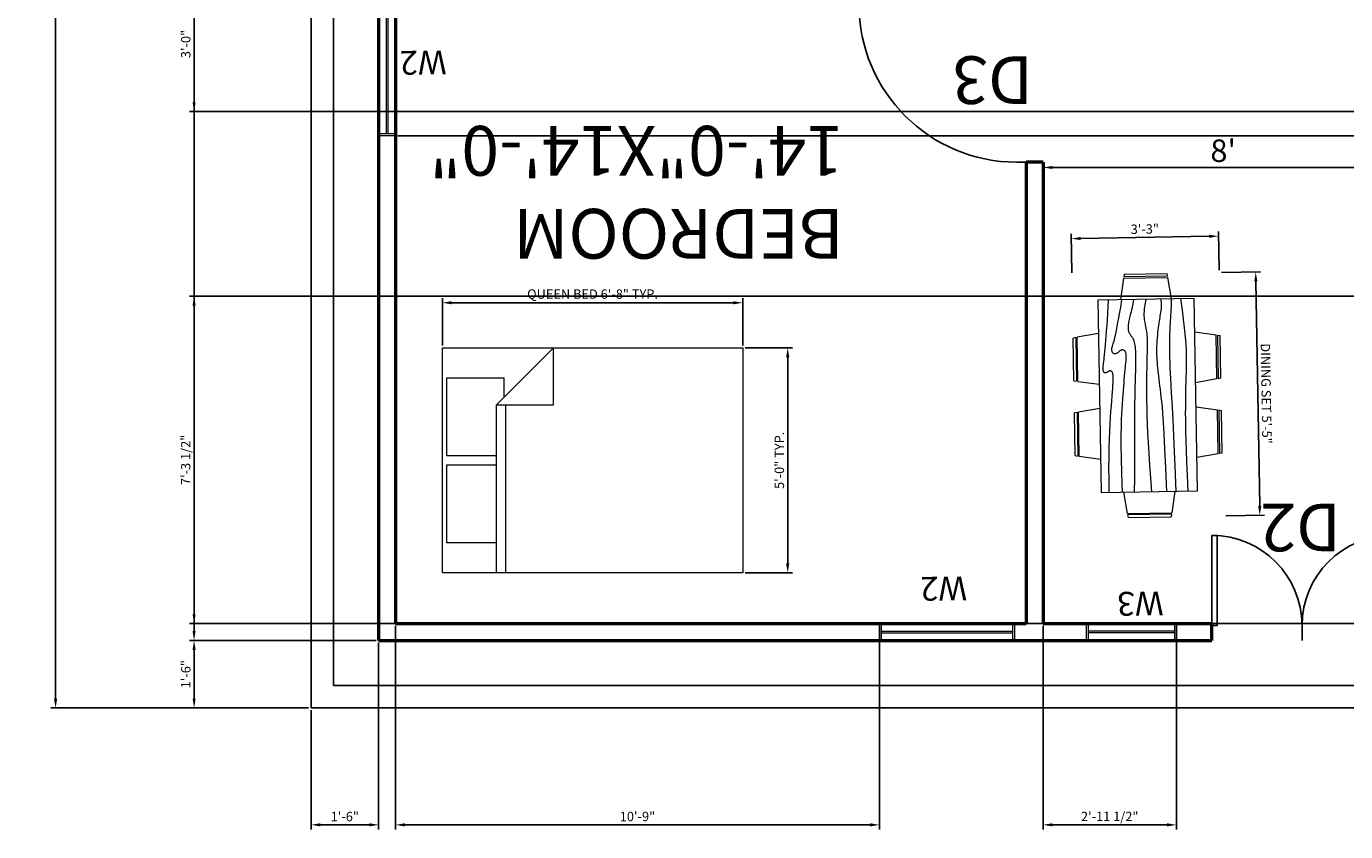
# Model space of a CAD drawing. Units: inches. Extents: x 1989 to 2637, y 1032 to 1611.
# Tile 1 of 5: x 1989 to 2340, y 1032 to 1247. Entities that reach past the tile are written whole.
import ezdxf

# ---------------------------------------------------------------- set-up
doc = ezdxf.new("R2010")
doc.units = ezdxf.units.IN
for name, color, linetype, lineweight in [('A-ANNO-TEXT', 1, 'Continuous', 18), ('A-AREA-IDEN', 1, 'Continuous', 25), ('C-PROP', 7, 'Continuous', 25), ('DIMENSIONS', 7, 'Continuous', 18), ('doors', 5, 'Continuous', 25), ('furniture', 8, 'Continuous', 18), ('walls', 7, 'Continuous', 50), ('windows', 3, 'Continuous', 18)]:
    doc.layers.add(name, color=color, linetype=linetype, lineweight=lineweight)
doc.styles.get("Standard").update_dxf_attribs({"font": 'arial.ttf'})
doc.dimstyles.new('ISO-25', dxfattribs={"dimtxt": 2.5, "dimasz": 2.5, "dimexe": 1.25, "dimexo": 0.625, "dimtad": 1, "dimlunit": 4, "dimtxsty": 'Standard', "dimcen": 2.5, "dimadec": 0, "dimazin": 0, "dimtfac": 1, "dimtmove": 0, "dimatfit": 3, "dimfxl": 1, "dimarcsym": 0})

# ---------------------------------------------------------------- blocks, each defined once
blk = doc.blocks.new('*U2')
for p, q in [((0, 0), (0, -5)), ((30, 0), (30, -5))]:
    blk.add_line(p, q)
blk.add_lwpolyline([(0, 0), (0, 30), (1.75, 30), (1.75, 0)], close=True)
blk.add_arc((0, 0), 30, 0, 90)
blk = doc.blocks.new('Dining Set - 36 x 72 in.')
for p, q in [((-22.2343, 26.00059), (-23.4847, 17.99762)), ((-22.2304, 26), (-5.7608, 26)), ((-22, 27.5), (-22.1562, 26.50042)), ((-5.8416, 26.5), (-22.1534, 26.5)), ((-22, 27.5), (-6, 27.5)), ((-5.8437, 26.49966), (-6, 27.5)), ((-4.5152, 17.99762), (-5.7655, 25.99926)), ((5.7657, 26.00059), (4.5153, 17.99762)), ((5.7696, 26), (22.2392, 26)), ((6, 27.5), (5.8438, 26.50042)), ((22.1584, 26.5), (5.8466, 26.5)), ((6, 27.5), (22, 27.5)), ((22.1563, 26.49966), (22, 27.5)), ((23.4848, 17.99762), (22.2345, 25.99926)), ((36, 18), (-36, 18)), ((-36, 18), (-36, -18)), ((36, -18), (36, 18)), ((-45.5, 8), (-44.5004, 8.15617)), ((-45.5, 8), (-45.5, -8)), ((-44.5, -8.15843), (-44.5, 8.15338)), ((-44.0006, 8.23428), (-35.9976, 9.48474)), ((-44, 8.23041), (-44, -8.23915)), ((44.0006, 8.23428), (35.9976, 9.48474)), ((44, 8.23041), (44, -8.23915)), ((44.5, -8.15843), (44.5, 8.15338)), ((45.5, 8), (44.5005, 8.15617)), ((45.5, 8), (45.5, -8)), ((-44.4997, -8.15631), (-45.5, -8)), ((-35.9976, -9.48476), (-43.9993, -8.2345)), ((35.9976, -9.48476), (43.9993, -8.2345)), ((44.4997, -8.15631), (45.5, -8)), ((-36, -18), (36, -18)), ((-22.2343, -26.0006), (-23.4847, -17.99762)), ((-4.5152, -17.99762), (-5.7655, -25.99928)), ((5.7657, -26.0006), (4.5153, -17.99762)), ((23.4848, -17.99762), (22.2345, -25.99928)), ((-22.2304, -26), (-5.7608, -26)), ((-22, -27.5), (-22.1562, -26.50044)), ((-5.8416, -26.5), (-22.1534, -26.5)), ((-22, -27.5), (-6, -27.5)), ((-5.8437, -26.49967), (-6, -27.5)), ((5.7696, -26), (22.2392, -26)), ((6, -27.5), (5.8438, -26.50044)), ((22.1584, -26.5), (5.8466, -26.5)), ((6, -27.5), (22, -27.5)), ((22.1563, -26.49967), (22, -27.5))]:
    blk.add_line(p, q)
for points in [[(-36, 15), (-31.1772, 14.97754), (-26.8079, 14.91406), (-22.8538, 14.81543), (-19.276, 14.6875), (-16.0362, 14.53613), (-13.0957, 14.36718), (-10.4159, 14.18652), (-7.9583, 14), (-5.6904, 13.81315), (-3.6035, 13.63021), (-1.6954, 13.45508), (0.0365, 13.29166), (1.5945, 13.14388), (2.9811, 13.01562), (4.1988, 12.9108), (5.25, 12.83333), (6.1393, 12.78613), (6.8802, 12.76823), (7.4883, 12.77767), (7.9792, 12.8125), (8.3685, 12.87077), (8.6719, 12.95052), (8.9049, 13.0498), (9.0833, 13.16666), (9.2205, 13.29899), (9.3216, 13.44401), (9.3895, 13.59879), (9.4271, 13.76041), (9.4373, 13.92594), (9.4232, 14.09245), (9.3875, 14.257), (9.3333, 14.41666), (9.2638, 14.56917), (9.1836, 14.71484), (9.0975, 14.85465), (9.0104, 14.98958), (8.9272, 15.1206), (8.8529, 15.2487), (8.7922, 15.37483), (8.75, 15.5), (8.7305, 15.62467), (8.7344, 15.74739), (8.7617, 15.86621), (8.8125, 15.97916), (8.8867, 16.08431), (8.9844, 16.17968), (9.1055, 16.26334), (9.25, 16.33333), (9.4189, 16.38802), (9.6172, 16.42708), (9.8506, 16.45052), (10.125, 16.45833), (10.4463, 16.45052), (10.8203, 16.42708), (11.2529, 16.38802), (11.75, 16.33333), (12.3184, 16.26318), (12.9694, 16.17838), (13.7151, 16.07991), (14.5677, 15.96875), (15.5395, 15.84586), (16.6426, 15.71224), (17.8893, 15.56884), (19.2917, 15.41666), (20.859, 15.25667), (22.5879, 15.08984), (24.4721, 14.91715), (26.5052, 14.73958), (28.6809, 14.5581), (30.9929, 14.3737), (33.4347, 14.18733), (36, 14)], [(-36, 10), (-28.9766, 10.14274), (-23.1725, 10.20442), (-18.4241, 10.19775), (-14.5677, 10.13541), (-11.4399, 10.03011), (-8.877, 9.89453), (-6.7154, 9.74137), (-4.7917, 9.58333), (-2.9698, 9.43082), (-1.2246, 9.28515), (0.4415, 9.14534), (2.026, 9.01041), (3.5266, 8.87939), (4.9408, 8.7513), (6.266, 8.62516), (7.5, 8.5), (8.6411, 8.37549), (9.6914, 8.2539), (10.6538, 8.13818), (11.5312, 8.03125), (12.3267, 7.93603), (13.043, 7.85547), (13.6831, 7.79248), (14.25, 7.75), (14.7471, 7.7303), (15.1797, 7.73307), (15.5537, 7.75732), (15.875, 7.80208), (16.1494, 7.86637), (16.3828, 7.94922), (16.5811, 8.04964), (16.75, 8.16666), (16.8944, 8.29915), (17.0143, 8.44531), (17.1089, 8.60319), (17.1771, 8.77083), (17.218, 8.94629), (17.2305, 9.1276), (17.2137, 9.31282), (17.1667, 9.5), (17.0895, 9.6875), (16.987, 9.875), (16.8649, 10.0625), (16.7292, 10.25), (16.5856, 10.4375), (16.4401, 10.625), (16.2985, 10.8125), (16.1667, 11), (16.05, 11.18733), (15.9518, 11.3737), (15.8752, 11.5581), (15.8229, 11.73958), (15.798, 11.91715), (15.8034, 12.08984), (15.842, 12.25667), (15.9167, 12.41666), (16.0295, 12.56836), (16.1784, 12.70833), (16.3605, 12.83268), (16.5729, 12.9375), (16.8127, 13.01888), (17.0768, 13.07291), (17.3625, 13.0957), (17.6667, 13.08333), (17.9894, 13.03312), (18.3418, 12.94726), (18.7382, 12.82918), (19.1927, 12.68229), (19.7195, 12.51001), (20.3327, 12.31575), (21.0465, 12.10294), (21.875, 11.875), (22.8357, 11.63354), (23.959, 11.37304), (25.2786, 11.08618), (26.8282, 10.76562), (28.6414, 10.40405), (30.752, 9.99414), (33.1936, 9.52856), (36, 9)], [(-36, 5.5), (-30.7157, 5.3348), (-26.069, 5.20963), (-21.9946, 5.11767), (-18.4271, 5.05208), (-15.3009, 5.00602), (-12.5508, 4.97265), (-10.1112, 4.94515), (-7.9167, 4.91666), (-5.909, 4.88167), (-4.0586, 4.83984), (-2.3429, 4.79215), (-0.7396, 4.73958), (0.7739, 4.6831), (2.22, 4.6237), (3.6213, 4.56233), (5, 4.5), (6.373, 4.43782), (7.7344, 4.3776), (9.0723, 4.32129), (10.375, 4.27083), (11.6309, 4.22819), (12.8281, 4.19531), (13.9551, 4.17415), (15, 4.16666), (15.954, 4.17448), (16.819, 4.19791), (17.6001, 4.23698), (18.3021, 4.29166), (18.9299, 4.36198), (19.4883, 4.44791), (19.9823, 4.54948), (20.4167, 4.66666), (20.7969, 4.79899), (21.1302, 4.94401), (21.4245, 5.09879), (21.6875, 5.26041), (21.9271, 5.42594), (22.1511, 5.59245), (22.3672, 5.757), (22.5834, 5.91666), (22.8065, 6.06868), (23.0404, 6.21093), (23.2879, 6.34147), (23.5521, 6.45833), (23.8358, 6.55957), (24.142, 6.64323), (24.4735, 6.70735), (24.8334, 6.75), (25.2235, 6.76969), (25.642, 6.76692), (26.0858, 6.74267), (26.5521, 6.69791), (27.0379, 6.63362), (27.5404, 6.55078), (28.0565, 6.45036), (28.5834, 6.33333), (29.1242, 6.19987), (29.7071, 6.04687), (30.3661, 5.87044), (31.1354, 5.66666), (32.0493, 5.43164), (33.142, 5.16146), (34.4475, 4.85221), (36, 4.5)], [(-36, -1), (-30.7915, -0.6591), (-26.0195, -0.38216), (-21.6519, -0.16284), (-17.6563, 0.00521), (-14.0005, 0.12833), (-10.6523, 0.21289), (-7.5796, 0.26522), (-4.75, 0.29166), (-2.134, 0.29793), (0.2878, 0.28711), (2.5317, 0.26163), (4.6146, 0.22396), (6.5529, 0.17651), (8.3633, 0.12174), (10.0623, 0.06209), (11.6667, 0), (13.1899, -0.06201), (14.6341, -0.1211), (15.9982, -0.17432), (17.2813, -0.21875), (18.4823, -0.25147), (19.6003, -0.26953), (20.6343, -0.27002), (21.5834, -0.25), (22.4481, -0.20768), (23.2357, -0.14584), (23.9549, -0.06836), (24.6146, 0.02083), (25.2235, 0.11784), (25.7904, 0.21875), (26.3241, 0.31966), (26.8334, 0.41666), (27.3265, 0.50618), (27.8099, 0.58593), (28.2894, 0.65397), (28.7709, 0.70833), (29.2601, 0.74707), (29.763, 0.76823), (30.2855, 0.76985), (30.8334, 0.75), (31.4088, 0.70784), (31.9994, 0.64713), (32.589, 0.57275), (33.1615, 0.48958), (33.7008, 0.4025), (34.1908, 0.3164), (34.6153, 0.23616), (34.9584, 0.16666), (35.2099, 0.11165), (35.3848, 0.07031), (35.504, 0.04069), (35.5886, 0.02083), (35.6594, 0.00879), (35.7377, 0.0026), (35.8442, 0.00032), (36, 0)], [(-36, -6.5), (-27.1843, -6.31267), (-20.084, -6.1263), (-14.469, -5.9419), (-10.1094, -5.76042), (-6.7752, -5.58285), (-4.2363, -5.41016), (-2.2629, -5.24333), (-0.625, -5.08334), (0.8708, -4.93099), (2.2715, -4.78646), (3.5872, -4.64974), (4.8281, -4.52084), (6.0046, -4.39974), (7.127, -4.28646), (8.2053, -4.18099), (9.25, -4.08334), (10.2705, -3.99382), (11.2734, -3.91407), (12.2647, -3.84603), (13.25, -3.79167), (14.2354, -3.75293), (15.2266, -3.73177), (16.2295, -3.73015), (17.25, -3.75), (18.2912, -3.79248), (19.3451, -3.85547), (20.4009, -3.93604), (21.4479, -4.03125), (22.4754, -4.13819), (23.4727, -4.25391), (24.4289, -4.37549), (25.3334, -4.5), (26.1785, -4.62492), (26.9694, -4.74935), (27.7145, -4.87281), (28.4219, -4.99479), (29.1, -5.11483), (29.7572, -5.23242), (30.4016, -5.34709), (31.0417, -5.45834), (31.6837, -5.56437), (32.3262, -5.65821), (32.9658, -5.73153), (33.599, -5.77604), (34.2224, -5.78345), (34.8327, -5.74545), (35.4264, -5.65373), (36, -5.5)], [(-36, -10), (-26.4022, -9.81299), (-18.4675, -9.62891), (-11.9839, -9.45069), (-6.7396, -9.28125), (-2.5226, -9.12354), (0.8789, -8.98047), (3.6769, -8.85498), (6.0833, -8.75), (8.2767, -8.66765), (10.3021, -8.60677), (12.1712, -8.56543), (13.8958, -8.54167), (15.4876, -8.53353), (16.9583, -8.53907), (18.3197, -8.55632), (19.5834, -8.58334), (20.7616, -8.61841), (21.8685, -8.66081), (22.9188, -8.71004), (23.9271, -8.76563), (24.9081, -8.82707), (25.8763, -8.89388), (26.8465, -8.96558), (27.8334, -9.04167), (28.8474, -9.12118), (29.8828, -9.20117), (30.93, -9.27824), (31.9792, -9.34896), (33.0205, -9.40991), (34.0443, -9.45768), (35.0407, -9.48885), (36, -9.5)], [(-36, -14.5), (-30.0881, -14.33513), (-25.0332, -14.21224), (-20.7312, -14.12647), (-17.0781, -14.07292), (-13.97, -14.04671), (-11.3027, -14.04297), (-8.9724, -14.05681), (-6.875, -14.08334), (-4.9224, -14.11833), (-3.0905, -14.16016), (-1.3709, -14.20785), (0.2448, -14.26042), (1.7647, -14.3169), (3.1973, -14.3763), (4.5507, -14.43767), (5.8333, -14.5), (7.0554, -14.5621), (8.235, -14.62175), (9.3922, -14.67652), (10.5469, -14.72396), (11.7192, -14.76164), (12.929, -14.78711), (14.1965, -14.79794), (15.5417, -14.79167), (16.9933, -14.76424), (18.6152, -14.70508), (20.4804, -14.60197), (22.6615, -14.44271), (25.2312, -14.21509), (28.2624, -13.9069), (31.8277, -13.50594), (36, -13)]]:
    blk.add_lwpolyline(points)
blk = doc.blocks.new('Bed - Queen')
for p, q in [((0, -80.00003), (0, 0)), ((0, 0), (59.99999, 0)), ((59.99999, 0), (59.99999, -80.00003)), ((7.99999, -1.2), (28.79998, -1.2)), ((7.99999, -14.4), (7.99999, -1.2)), ((28.79998, -1.2), (28.79998, -14.4)), ((31.19999, -1.2), (51.99999, -1.2)), ((31.19999, -14.4), (31.19999, -1.2)), ((51.99999, -1.2), (51.99999, -16.4)), ((0, -14.4), (44.8, -14.4)), ((44.8, -16.8), (0, -16.8)), ((59.99999, -29.6), (44.8, -14.4)), ((44.8, -14.4), (44.8, -29.6)), ((51.99999, -16.4), (46.79936, -16.4)), ((44.8, -29.6), (59.99999, -29.6)), ((59.99999, -80.00003), (0, -80.00003))]:
    blk.add_line(p, q)
blk = doc.blocks.new('*D11')
at = {"layer": 'Defpoints', "color": 0, "transparency": 16777216}
for p in [(1996.45, 1544.92), (2064.5, 1544.92), (2064.5, 1064.92)]:
    blk.add_point(p, dxfattribs=at)
at = {"layer": 'DIMENSIONS', "color": 0, "lineweight": -2, "transparency": 16777216}
for p, q in [((2063.87, 1544.92), (1995.2, 1544.92)), ((1996.45, 1067.42), (1996.45, 1542.42)), ((2063.87, 1064.92), (1995.2, 1064.92))]:
    blk.add_line(p, q, dxfattribs=at)
at = {"layer": 'DIMENSIONS', "color": 0, "transparency": 16777216}
for points in [[(1996.03, 1542.42), (1996.87, 1542.42), (1996.45, 1544.92)], [(1996.03, 1067.42), (1996.87, 1067.42), (1996.45, 1064.92)]]:
    blk.add_solid(points, dxfattribs=at)
at = {"layer": 'DIMENSIONS', "color": 0, "transparency": 16777216, "insert": (1992.76, 1304.92), "char_height": 6, "attachment_point": 5, "rotation": 90}
blk.add_mtext("40'", dxfattribs=at)
blk = doc.blocks.new('*D16')
at = {"layer": 'Defpoints', "color": 0, "transparency": 16777216}
for p in [(2259.5, 1209.01), (2259.5, 1190.91), (2355.5, 1190.91)]:
    blk.add_point(p, dxfattribs=at)
at = {"layer": 'DIMENSIONS', "color": 0, "lineweight": -2, "transparency": 16777216}
for p, q in [((2259.5, 1191.53), (2259.5, 1210.26)), ((2353, 1209.01), (2262, 1209.01)), ((2355.5, 1191.53), (2355.5, 1210.26))]:
    blk.add_line(p, q, dxfattribs=at)
at = {"layer": 'DIMENSIONS', "color": 0, "transparency": 16777216}
for points in [[(2262, 1209.43), (2262, 1208.6), (2259.5, 1209.01)], [(2353, 1209.43), (2353, 1208.6), (2355.5, 1209.01)]]:
    blk.add_solid(points, dxfattribs=at)
at = {"layer": 'DIMENSIONS', "color": 0, "transparency": 16777216, "insert": (2307.5, 1212.7), "char_height": 6, "attachment_point": 5}
blk.add_mtext("8'", dxfattribs=at)
blk = doc.blocks.new('WIN-W3-24IN')
for p, q in [((0, 0), (0, 23.95)), ((0, 23.95), (4.5, 23.95)), ((0, 23.45), (4.5, 23.45)), ((2.05, 23.45), (2.05, 0.5)), ((2.45, 23.45), (2.45, 0.5)), ((4.5, 23.95), (4.5, 0)), ((4.5, 0.5), (0, 0.5)), ((4.5, 0), (0, 0))]:
    blk.add_line(p, q)
blk = doc.blocks.new('WIN-W2-36IN')
for p, q in [((0, 0), (0, 35.95)), ((0, 35.95), (4.5, 35.95)), ((0, 35.45), (4.5, 35.45)), ((2.05, 35.45), (2.05, 0.5)), ((2.45, 35.45), (2.45, 0.5)), ((4.5, 35.95), (4.5, 0)), ((4.5, 0.5), (0, 0.5)), ((4.5, 0), (0, 0))]:
    blk.add_line(p, q)
blk = doc.blocks.new('*D30')
at = {"layer": 'Defpoints', "color": 0, "transparency": 16777216}
for p in [(2099.49, 1172.94), (2099.49, 1160.94), (2179.49, 1160.94)]:
    blk.add_point(p, dxfattribs=at)
at = {"layer": 'DIMENSIONS', "color": 0, "lineweight": -2, "transparency": 16777216}
for p, q in [((2099.49, 1161.57), (2099.49, 1174.19)), ((2179.49, 1161.57), (2179.49, 1174.19)), ((2176.99, 1172.94), (2101.99, 1172.94))]:
    blk.add_line(p, q, dxfattribs=at)
at = {"layer": 'DIMENSIONS', "color": 0, "transparency": 16777216}
for points in [[(2101.99, 1173.36), (2101.99, 1172.53), (2099.49, 1172.94)], [(2176.99, 1173.36), (2176.99, 1172.53), (2179.49, 1172.94)]]:
    blk.add_solid(points, dxfattribs=at)
at = {"layer": 'DIMENSIONS', "color": 0, "transparency": 16777216, "insert": (2139.49, 1174.94), "char_height": 2.5, "attachment_point": 5}
blk.add_mtext('QUEEN BED 6\'-8" TYP.', dxfattribs=at)
blk = doc.blocks.new('*D31')
at = {"layer": 'Defpoints', "color": 0, "transparency": 16777216}
for p in [(2179.49, 1160.94), (2191.49, 1160.94), (2179.49, 1100.94)]:
    blk.add_point(p, dxfattribs=at)
at = {"layer": 'DIMENSIONS', "color": 0, "lineweight": -2, "transparency": 16777216}
for p, q in [((2180.11, 1160.94), (2192.74, 1160.94)), ((2191.49, 1103.44), (2191.49, 1158.44)), ((2180.11, 1100.94), (2192.74, 1100.94))]:
    blk.add_line(p, q, dxfattribs=at)
at = {"layer": 'DIMENSIONS', "color": 0, "transparency": 16777216}
for points in [[(2191.07, 1158.44), (2191.9, 1158.44), (2191.49, 1160.94)], [(2191.07, 1103.44), (2191.9, 1103.44), (2191.49, 1100.94)]]:
    blk.add_solid(points, dxfattribs=at)
at = {"layer": 'DIMENSIONS', "color": 0, "transparency": 16777216, "insert": (2189.59, 1130.94), "char_height": 2.5, "attachment_point": 5, "rotation": 90}
blk.add_mtext('5\'-0" TYP.', dxfattribs=at)
blk = doc.blocks.new('*D34')
at = {"layer": 'Defpoints', "color": 0, "transparency": 16777216}
for p in [(2306.43, 1180.97), (2316.16, 1181.14), (2307.53, 1116.11)]:
    blk.add_point(p, dxfattribs=at)
at = {"layer": 'DIMENSIONS', "color": 0, "lineweight": -2, "transparency": 16777216}
for p, q in [((2307.05, 1180.98), (2317.41, 1181.16)), ((2317.22, 1118.78), (2316.2, 1178.64)), ((2308.16, 1116.12), (2318.51, 1116.3))]:
    blk.add_line(p, q, dxfattribs=at)
at = {"layer": 'DIMENSIONS', "color": 0, "transparency": 16777216}
for points in [[(2316.62, 1178.64), (2315.78, 1178.63), (2316.16, 1181.14)], [(2317.64, 1118.78), (2316.8, 1118.77), (2317.26, 1116.28)]]:
    blk.add_solid(points, dxfattribs=at)
at = {"layer": 'DIMENSIONS', "color": 0, "transparency": 16777216, "insert": (2318.63, 1148.74), "char_height": 2.5, "attachment_point": 5, "rotation": 270.9757}
blk.add_mtext('DINING SET 5\'-5"', dxfattribs=at)
blk = doc.blocks.new('*D35')
at = {"layer": 'Defpoints', "color": 0, "transparency": 16777216}
for p in [(2267.06, 1190.03), (2306.43, 1180.97), (2267.23, 1180.3)]:
    blk.add_point(p, dxfattribs=at)
at = {"layer": 'DIMENSIONS', "color": 0, "lineweight": -2, "transparency": 16777216}
for p, q in [((2306.42, 1181.6), (2306.24, 1191.95)), ((2267.22, 1180.93), (2267.04, 1191.28)), ((2303.76, 1190.66), (2269.56, 1190.07))]:
    blk.add_line(p, q, dxfattribs=at)
at = {"layer": 'DIMENSIONS', "color": 0, "transparency": 16777216}
for points in [[(2269.55, 1190.49), (2269.57, 1189.66), (2267.06, 1190.03)], [(2303.76, 1191.07), (2303.77, 1190.24), (2306.26, 1190.7)]]:
    blk.add_solid(points, dxfattribs=at)
at = {"layer": 'DIMENSIONS', "color": 0, "transparency": 16777216, "insert": (2286.63, 1192.27), "char_height": 2.5, "attachment_point": 5, "rotation": 0.9757}
blk.add_mtext('3\'-3"', dxfattribs=at)
blk = doc.blocks.new('*D41')
at = {"layer": 'Defpoints', "color": 0, "transparency": 16777216}
for p in [(2033.35, 1496.92), (2082.5, 1496.92), (2082.5, 1082.92)]:
    blk.add_point(p, dxfattribs=at)
at = {"layer": 'DIMENSIONS', "color": 0, "lineweight": -2, "transparency": 16777216}
for p, q in [((2081.87, 1496.92), (2032.1, 1496.92)), ((2033.35, 1085.42), (2033.35, 1494.42)), ((2081.87, 1082.92), (2032.1, 1082.92))]:
    blk.add_line(p, q, dxfattribs=at)
at = {"layer": 'DIMENSIONS', "color": 0, "transparency": 16777216}
for points in [[(2032.93, 1494.42), (2033.76, 1494.42), (2033.35, 1496.92)], [(2032.93, 1085.42), (2033.76, 1085.42), (2033.35, 1082.92)]]:
    blk.add_solid(points, dxfattribs=at)
at = {"layer": 'DIMENSIONS', "color": 0, "transparency": 16777216, "insert": (2031.45, 1289.92), "char_height": 2.5, "attachment_point": 5, "rotation": 90}
blk.add_mtext('34\'-6"', dxfattribs=at)
blk = doc.blocks.new('*D52')
at = {"layer": 'Defpoints', "color": 0, "transparency": 16777216}
for p in [(2082.5, 1082.92), (2064.5, 1064.92), (2082.5, 1033.77)]:
    blk.add_point(p, dxfattribs=at)
at = {"layer": 'DIMENSIONS', "color": 0, "lineweight": -2, "transparency": 16777216}
for p, q in [((2082.5, 1082.3), (2082.5, 1032.52)), ((2064.5, 1064.3), (2064.5, 1032.52)), ((2067, 1033.77), (2080, 1033.77))]:
    blk.add_line(p, q, dxfattribs=at)
at = {"layer": 'DIMENSIONS', "color": 0, "transparency": 16777216}
for points in [[(2067, 1034.19), (2067, 1033.35), (2064.5, 1033.77)], [(2080, 1034.19), (2080, 1033.35), (2082.5, 1033.77)]]:
    blk.add_solid(points, dxfattribs=at)
at = {"layer": 'DIMENSIONS', "color": 0, "transparency": 16777216, "insert": (2073.5, 1035.67), "char_height": 2.5, "attachment_point": 5}
blk.add_mtext('1\'-6"', dxfattribs=at)
blk = doc.blocks.new('*D53')
at = {"layer": 'Defpoints', "color": 0, "transparency": 16777216}
for p in [(2033.35, 1082.92), (2082.5, 1082.92), (2064.5, 1064.92)]:
    blk.add_point(p, dxfattribs=at)
at = {"layer": 'DIMENSIONS', "color": 0, "lineweight": -2, "transparency": 16777216}
for p, q in [((2081.87, 1082.92), (2032.1, 1082.92)), ((2033.35, 1067.42), (2033.35, 1080.42)), ((2063.87, 1064.92), (2032.1, 1064.92))]:
    blk.add_line(p, q, dxfattribs=at)
at = {"layer": 'DIMENSIONS', "color": 0, "transparency": 16777216}
for points in [[(2032.93, 1080.42), (2033.76, 1080.42), (2033.35, 1082.92)], [(2032.93, 1067.42), (2033.76, 1067.42), (2033.35, 1064.92)]]:
    blk.add_solid(points, dxfattribs=at)
at = {"layer": 'DIMENSIONS', "color": 0, "transparency": 16777216, "insert": (2031.45, 1073.92), "char_height": 2.5, "attachment_point": 5, "rotation": 90}
blk.add_mtext('1\'-6"', dxfattribs=at)
blk = doc.blocks.new('*D59')
at = {"layer": 'Defpoints', "color": 0, "transparency": 16777216}
for p in [(2033.35, 1259.92), (2415.5, 1259.92), (2415.5, 1223.92)]:
    blk.add_point(p, dxfattribs=at)
at = {"layer": 'DIMENSIONS', "color": 0, "lineweight": -2, "transparency": 16777216}
for p, q in [((2414.87, 1259.92), (2032.1, 1259.92)), ((2033.35, 1226.42), (2033.35, 1257.42)), ((2414.87, 1223.92), (2032.1, 1223.92))]:
    blk.add_line(p, q, dxfattribs=at)
at = {"layer": 'DIMENSIONS', "color": 0, "transparency": 16777216}
for points in [[(2032.93, 1257.42), (2033.76, 1257.42), (2033.35, 1259.92)], [(2032.93, 1226.42), (2033.76, 1226.42), (2033.35, 1223.92)]]:
    blk.add_solid(points, dxfattribs=at)
at = {"layer": 'DIMENSIONS', "color": 0, "transparency": 16777216, "insert": (2031.45, 1241.92), "char_height": 2.5, "attachment_point": 5, "rotation": 90}
blk.add_mtext('3\'-0"', dxfattribs=at)
blk = doc.blocks.new('*D61')
at = {"layer": 'Defpoints', "color": 0, "transparency": 16777216}
for p in [(2033.35, 1174.7), (2480, 1174.7), (2480, 1087.42)]:
    blk.add_point(p, dxfattribs=at)
at = {"layer": 'DIMENSIONS', "color": 0, "lineweight": -2, "transparency": 16777216}
for p, q in [((2479.37, 1174.7), (2032.1, 1174.7)), ((2033.35, 1089.92), (2033.35, 1172.2)), ((2479.37, 1087.42), (2032.1, 1087.42))]:
    blk.add_line(p, q, dxfattribs=at)
at = {"layer": 'DIMENSIONS', "color": 0, "transparency": 16777216}
for points in [[(2032.93, 1172.2), (2033.76, 1172.2), (2033.35, 1174.7)], [(2032.93, 1089.92), (2033.76, 1089.92), (2033.35, 1087.42)]]:
    blk.add_solid(points, dxfattribs=at)
at = {"layer": 'DIMENSIONS', "color": 0, "transparency": 16777216, "insert": (2031.43, 1131.06), "char_height": 2.5, "attachment_point": 5, "rotation": 90}
blk.add_mtext('7\'-3 1/2"', dxfattribs=at)
blk = doc.blocks.new('*D62')
at = {"layer": 'Defpoints', "color": 0, "transparency": 16777216}
for p in [(2086.98, 1217.46), (2635.65, 1217.46), (2087, 1087.42)]:
    blk.add_point(p, dxfattribs=at)
at = {"layer": 'DIMENSIONS', "color": 0, "lineweight": -2, "transparency": 16777216}
for p, q in [((2087.6, 1217.46), (2636.9, 1217.46)), ((2635.65, 1089.92), (2635.65, 1214.96)), ((2087.62, 1087.42), (2636.9, 1087.42))]:
    blk.add_line(p, q, dxfattribs=at)
at = {"layer": 'DIMENSIONS', "color": 0, "transparency": 16777216}
for points in [[(2635.23, 1214.96), (2636.06, 1214.96), (2635.65, 1217.46)], [(2635.23, 1089.92), (2636.06, 1089.92), (2635.65, 1087.42)]]:
    blk.add_solid(points, dxfattribs=at)
at = {"layer": 'DIMENSIONS', "color": 0, "transparency": 16777216, "insert": (2633.75, 1152.44), "char_height": 2.5, "attachment_point": 5, "rotation": 90}
blk.add_mtext('10\'-10"', dxfattribs=at)
blk = doc.blocks.new('*D64')
at = {"layer": 'Defpoints', "color": 0, "transparency": 16777216}
for p in [(2259.5, 1087.42), (2295.05, 1087.42), (2295.05, 1033.77)]:
    blk.add_point(p, dxfattribs=at)
at = {"layer": 'DIMENSIONS', "color": 0, "lineweight": -2, "transparency": 16777216}
for p, q in [((2259.5, 1086.8), (2259.5, 1032.52)), ((2295.05, 1086.8), (2295.05, 1032.52)), ((2262, 1033.77), (2292.55, 1033.77))]:
    blk.add_line(p, q, dxfattribs=at)
at = {"layer": 'DIMENSIONS', "color": 0, "transparency": 16777216}
for points in [[(2262, 1034.19), (2262, 1033.35), (2259.5, 1033.77)], [(2292.55, 1034.19), (2292.55, 1033.35), (2295.05, 1033.77)]]:
    blk.add_solid(points, dxfattribs=at)
at = {"layer": 'DIMENSIONS', "color": 0, "transparency": 16777216, "insert": (2277.27, 1035.69), "char_height": 2.5, "attachment_point": 5}
blk.add_mtext('2\'-11 1/2"', dxfattribs=at)
blk = doc.blocks.new('*D65')
at = {"layer": 'Defpoints', "color": 0, "transparency": 16777216}
for p in [(2087, 1087.42), (2215.93, 1087.42), (2215.93, 1033.77)]:
    blk.add_point(p, dxfattribs=at)
at = {"layer": 'DIMENSIONS', "color": 0, "lineweight": -2, "transparency": 16777216}
for p, q in [((2087, 1086.8), (2087, 1032.52)), ((2215.93, 1086.8), (2215.93, 1032.52)), ((2089.5, 1033.77), (2213.43, 1033.77))]:
    blk.add_line(p, q, dxfattribs=at)
at = {"layer": 'DIMENSIONS', "color": 0, "transparency": 16777216}
for points in [[(2089.5, 1034.19), (2089.5, 1033.35), (2087, 1033.77)], [(2213.43, 1034.19), (2213.43, 1033.35), (2215.93, 1033.77)]]:
    blk.add_solid(points, dxfattribs=at)
at = {"layer": 'DIMENSIONS', "color": 0, "transparency": 16777216, "insert": (2151.46, 1035.67), "char_height": 2.5, "attachment_point": 5}
blk.add_mtext('10\'-9"', dxfattribs=at)

msp = doc.modelspace()

# ---------------------------------------------------------------- linework, layer by layer
at = {"layer": 'C-PROP'}
for p, q in [((2064.498, 1544.921), (2064.498, 1064.921)), ((2070.498, 1538.921), (2070.498, 1070.921)), ((2070.498, 1070.921), (2598.498, 1070.921)), ((2064.498, 1064.921), (2604.498, 1064.921))]:
    msp.add_line(p, q, dxfattribs=at)
at = {"layer": 'walls'}
for p, q in [((2082.498, 1432.504), (2082.498, 1082.921)), ((2086.998, 1255.421), (2086.998, 1087.421)), ((2259.498, 1210.421), (2254.998, 1210.421)), ((2254.998, 1210.421), (2254.998, 1087.421)), ((2259.498, 1210.421), (2259.498, 1087.421)), ((2086.998, 1087.421), (2254.998, 1087.421)), ((2259.498, 1087.421), (2304.498, 1087.421)), ((2304.498, 1082.921), (2304.498, 1087.421)), ((2082.498, 1082.921), (2304.498, 1082.921))]:
    msp.add_line(p, q, dxfattribs=at)

# ---------------------------------------------------------------- block references
at = {"layer": 'doors', "xscale": -1.399999999999999, "yscale": 1.399999999999999, "zscale": 1.399999999999999, "rotation": 90}
msp.add_blockref('*U2', (2252.498, 1252.421), dxfattribs=at)
at = {"layer": 'doors', "yscale": 0.8, "zscale": 0.8}
for p, xscale in [((2304.498, 1086.921), 0.8), ((2352.498, 1086.921), -0.8)]:
    msp.add_blockref('*U2', p, dxfattribs=dict(at, xscale=xscale))
at = {"layer": 'furniture', "xscale": 0.7128292820237097, "yscale": 0.7128292820237097, "zscale": 0.7128292820237097, "rotation": 90.97568858518098}
msp.add_blockref('Dining Set - 36 x 72 in.', (2287.38, 1148.207), dxfattribs=at)
at = {"layer": 'furniture', "rotation": 90}
msp.add_blockref('Bed - Queen', (2099.488, 1100.942), dxfattribs=at)
at = {"layer": 'windows'}
msp.add_blockref('WIN-W2-36IN', (2082.48, 1217.461), dxfattribs=at)
for name, p, rotation in [('WIN-W2-36IN', (2251.88, 1082.921), 89.99999999999812), ('WIN-W3-24IN', (2271.099, 1087.421), 269.9999999999951)]:
    msp.add_blockref(name, p, dxfattribs=dict(at, rotation=rotation))

# ---------------------------------------------------------------- texts
at = {"layer": 'A-ANNO-TEXT', "attachment_point": 1}
for s, width, gutter_width, heights, insert, char_height, rotation in [('W2', 5.29651, 31.753, [0], (2100.635, 1233.865), 6.3507, 180.67334), ('D3', 3.801, 63.542, [0], (2256.818, 1225.936), 12.7085, 180), ('D2', 3.801, 63.542, [12.761], (2338.896, 1106.695), 12.7085, 180), ('W2', 5.29651, 31.753, [0], (2239.279, 1093.644), 6.3507, 180.67334), ('W3', 5.29651, 31.753, [0], (2291.647, 1089.637), 6.3507, 180.67334)]:
    msp.add_mtext_dynamic_manual_height_columns(s, width=width, gutter_width=gutter_width, heights=heights, dxfattribs=dict(at, insert=insert, char_height=char_height, rotation=rotation))
at = {"layer": 'A-AREA-IDEN', "insert": (2206.426, 1184.704), "char_height": 13.26964, "attachment_point": 1, "rotation": 180}
msp.add_mtext_dynamic_manual_height_columns('BEDROOM\\P14\'-0"X14\'-0"', width=13.72319, gutter_width=66.348, heights=[0], dxfattribs=at)

# ---------------------------------------------------------------- dimensions: what is measured, and where the dimension line sits
at = {"layer": 'DIMENSIONS'}
for base, p1, p2, angle, override, picture, middle in [((1996.449, 1544.921), (2064.498, 1064.921), (2064.498, 1544.921), 90, {"dimtxt": 6, "dimclrd": 0, "dimclre": 0, "dimclrt": 0}, '*D11', (1992.76, 1304.921)), ((2033.348, 1496.921), (2082.498, 1082.921), (2082.498, 1496.921), 90, {"dimdec": 1, "dimlfac": 1, "dimrnd": 0, "dimzin": 1, "dimdsep": 46, "dimlunit": 4, "dimfrac": 2}, '*D41', (2031.445, 1289.921)), ((2033.348, 1259.921), (2415.498, 1223.921), (2415.498, 1259.921), 90, {"dimdec": 1, "dimlfac": 1, "dimrnd": 0, "dimzin": 1, "dimdsep": 46, "dimlunit": 4, "dimfrac": 2}, '*D59', (2031.445, 1241.921)), ((2635.648, 1217.461), (2086.998, 1087.421), (2086.98, 1217.461), 90, {"dimdec": 1, "dimlfac": 1, "dimrnd": 0, "dimzin": 1, "dimdsep": 46, "dimlunit": 4, "dimfrac": 2}, '*D62', (2633.746, 1152.441)), ((2267.062, 1190.031), (2306.428, 1180.97), (2267.228, 1180.303), 180.97569, {"dimdec": 1, "dimlfac": 1, "dimrnd": 0, "dimzin": 1, "dimdsep": 46, "dimlunit": 4, "dimfrac": 2}, '*D35', (2286.63, 1192.267)), ((2033.348, 1174.701), (2479.998, 1087.421), (2479.998, 1174.701), 90, {"dimdec": 1, "dimlfac": 1, "dimrnd": 0, "dimzin": 1, "dimdsep": 46, "dimlunit": 4, "dimfrac": 2}, '*D61', (2031.429, 1131.061)), ((2033.348, 1082.921), (2064.498, 1064.921), (2082.498, 1082.921), 90, {"dimdec": 1, "dimlfac": 1, "dimrnd": 0, "dimzin": 1, "dimdsep": 46, "dimlunit": 4, "dimfrac": 2}, '*D53', (2031.446, 1073.921))]:
    dim = msp.add_linear_dim(base=base, p1=p1, p2=p2, angle=angle, dimstyle='ISO-25', override=override, dxfattribs=at)
    dim.commit()
    dim.dimension.update_dxf_attribs({"geometry": picture, "text_midpoint": middle})
for base, p1, p2, override, picture, middle in [((2259.498, 1209.015), (2355.498, 1190.907), (2259.498, 1190.907), {"dimtxt": 6, "dimclrd": 0, "dimclre": 0, "dimclrt": 0}, '*D16', (2307.498, 1212.703)), ((2215.93, 1033.771), (2086.998, 1087.421), (2215.93, 1087.421), {"dimdec": 1, "dimlfac": 1, "dimrnd": 0, "dimzin": 1, "dimdsep": 46, "dimlunit": 4, "dimfrac": 2}, '*D65', (2151.464, 1035.672)), ((2295.049, 1033.771), (2259.498, 1087.421), (2295.049, 1087.421), {"dimdec": 1, "dimlfac": 1, "dimrnd": 0, "dimzin": 1, "dimdsep": 46, "dimlunit": 4, "dimfrac": 2}, '*D64', (2277.273, 1035.689)), ((2082.498, 1033.771), (2064.498, 1064.921), (2082.498, 1082.921), {"dimdec": 1, "dimlfac": 1, "dimrnd": 0, "dimzin": 1, "dimdsep": 46, "dimlunit": 4, "dimfrac": 2}, '*D52', (2073.498, 1035.672))]:
    dim = msp.add_linear_dim(base=base, p1=p1, p2=p2, dimstyle='ISO-25', override=override, dxfattribs=at)
    dim.commit()
    dim.dimension.update_dxf_attribs({"geometry": picture, "text_midpoint": middle})
for base, p1, p2, angle, text, picture, middle in [((2099.488, 1172.942), (2179.488, 1160.942), (2099.488, 1160.942), 180, 'QUEEN BED <> TYP.', '*D30', (2139.488, 1174.936)), ((2316.157, 1181.136), (2307.532, 1116.112), (2306.428, 1180.97), 90.97569, 'DINING SET <>', '*D34', (2318.626, 1148.74)), ((2191.488, 1160.942), (2179.488, 1100.942), (2179.488, 1160.942), 90, '<> TYP.', '*D31', (2189.586, 1130.942))]:
    dim = msp.add_linear_dim(base=base, p1=p1, p2=p2, angle=angle, text=text, dimstyle='ISO-25', override={"dimdec": 1, "dimlfac": 1, "dimrnd": 0, "dimzin": 1, "dimdsep": 46, "dimlunit": 4, "dimfrac": 2}, dxfattribs=at)
    dim.commit()
    dim.dimension.update_dxf_attribs({"geometry": picture, "text_midpoint": middle})

doc.saveas('drawing.dxf')
